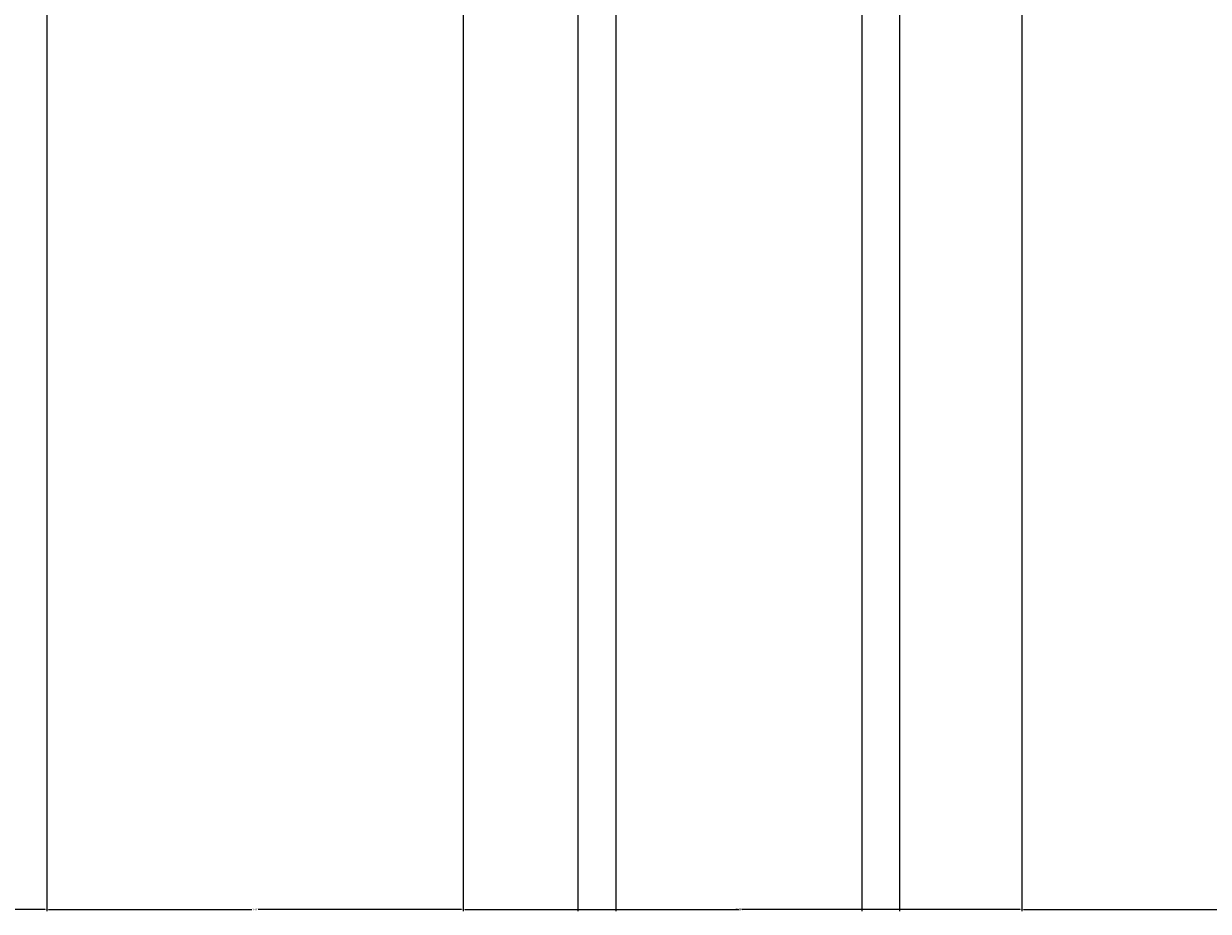
# Model space of a CAD drawing. Units: inches. Extents: x 37 to 824, y -700 to 234.
# Tile 9 of 77: x 253 to 378, y -700 to -606. Entities that reach past the tile are written whole.
import ezdxf

# ---------------------------------------------------------------- set-up
doc = ezdxf.new("R2010")
doc.units = ezdxf.units.IN
doc.header["$MEASUREMENT"] = 0
doc.layers.add('A-ANNO-DIMS', color=2, linetype='Continuous', lineweight=18)
doc.styles.get("Standard").update_dxf_attribs({"font": 'arial.ttf'})
doc.dimstyles.get("Standard").update_dxf_attribs({"dimtxt": 0.18, "dimasz": 0.18, "dimexe": 0.18, "dimexo": 0.0625, "dimgap": 0.09, "dimtad": 0, "dimtih": 1, "dimtoh": 1, "dimdec": 1, "dimzin": 0, "dimdsep": 46, "dimlunit": 4, "dimtxsty": 'Standard', "dimcen": 0.09, "dimadec": 0, "dimazin": 0, "dimtfac": 1, "dimtdec": 1, "dimtofl": 0, "dimtmove": 0, "dimatfit": 3, "dimfxl": 1, "dimtolj": 1, "dimtzin": 0, "dimarcsym": 0})

# ---------------------------------------------------------------- blocks, each defined once
blk = doc.blocks.new('*D68')
at = {"layer": 'A-ANNO-DIMS', "color": 0, "lineweight": -2, "ltscale": 0.5, "transparency": 16777216}
for p, q in [((205.08, -537.69), (205.08, -699.59)), ((255.08, -537.69), (255.08, -699.59)), ((205.26, -699.41), (229.74, -699.41)), ((254.9, -699.41), (230.41, -699.41))]:
    blk.add_line(p, q, dxfattribs=at)
at = {"layer": 'A-ANNO-DIMS', "color": 0, "ltscale": 0.5, "transparency": 16777216}
for points in [[(205.26, -699.38), (205.26, -699.44), (205.08, -699.41)], [(254.9, -699.38), (254.9, -699.44), (255.08, -699.41)]]:
    blk.add_solid(points, dxfattribs=at)
at = {"layer": 'Defpoints', "color": 0, "ltscale": 0.5, "transparency": 16777216}
for p in [(205.08, -537.63), (255.08, -537.63), (255.08, -699.41)]:
    blk.add_point(p, dxfattribs=at)
at = {"layer": 'A-ANNO-DIMS', "color": 0, "ltscale": 0.5, "transparency": 16777216, "insert": (230.08, -699.41), "char_height": 0.18, "attachment_point": 5}
blk.add_mtext('\\A1;4\'-2"', dxfattribs=at)
blk = doc.blocks.new('*D69')
at = {"layer": 'A-ANNO-DIMS', "color": 0, "lineweight": -2, "ltscale": 0.5, "transparency": 16777216}
for p, q in [((255.08, -537.69), (255.08, -699.59)), ((299.08, -585.69), (299.08, -699.59)), ((255.26, -699.41), (276.75, -699.41)), ((298.9, -699.41), (277.41, -699.41))]:
    blk.add_line(p, q, dxfattribs=at)
at = {"layer": 'A-ANNO-DIMS', "color": 0, "ltscale": 0.5, "transparency": 16777216}
for points in [[(255.26, -699.38), (255.26, -699.44), (255.08, -699.41)], [(298.9, -699.38), (298.9, -699.44), (299.08, -699.41)]]:
    blk.add_solid(points, dxfattribs=at)
at = {"layer": 'Defpoints', "color": 0, "ltscale": 0.5, "transparency": 16777216}
for p in [(255.08, -537.63), (299.08, -585.63), (299.08, -699.41)]:
    blk.add_point(p, dxfattribs=at)
at = {"layer": 'A-ANNO-DIMS', "color": 0, "ltscale": 0.5, "transparency": 16777216, "insert": (277.08, -699.41), "char_height": 0.18, "attachment_point": 5}
blk.add_mtext('\\A1;3\'-8"', dxfattribs=at)
blk = doc.blocks.new('*D70')
at = {"layer": 'A-ANNO-DIMS', "color": 0, "lineweight": -2, "ltscale": 0.5, "transparency": 16777216}
for p, q in [((299.08, -585.69), (299.08, -699.59)), ((358.13, -585.69), (358.13, -699.59)), ((299.26, -699.41), (328.2, -699.41)), ((357.95, -699.41), (329.01, -699.41))]:
    blk.add_line(p, q, dxfattribs=at)
at = {"layer": 'A-ANNO-DIMS', "color": 0, "ltscale": 0.5, "transparency": 16777216}
for points in [[(299.26, -699.38), (299.26, -699.44), (299.08, -699.41)], [(357.95, -699.38), (357.95, -699.44), (358.13, -699.41)]]:
    blk.add_solid(points, dxfattribs=at)
at = {"layer": 'Defpoints', "color": 0, "ltscale": 0.5, "transparency": 16777216}
for p in [(299.08, -585.63), (358.13, -585.63), (358.13, -699.41)]:
    blk.add_point(p, dxfattribs=at)
at = {"layer": 'A-ANNO-DIMS', "color": 0, "ltscale": 0.5, "transparency": 16777216, "insert": (328.6, -699.41), "char_height": 0.18, "attachment_point": 5}
blk.add_mtext('\\A1;4\'-11"', dxfattribs=at)
blk = doc.blocks.new('*D71')
at = {"layer": 'A-ANNO-DIMS', "color": 0, "lineweight": -2, "ltscale": 0.5, "transparency": 16777216}
for p, q in [((358.13, -585.69), (358.13, -699.59)), ((428.08, -585.69), (428.08, -699.59)), ((358.31, -699.41), (392.71, -699.41)), ((427.9, -699.41), (393.5, -699.41))]:
    blk.add_line(p, q, dxfattribs=at)
at = {"layer": 'A-ANNO-DIMS', "color": 0, "ltscale": 0.5, "transparency": 16777216}
for points in [[(358.31, -699.38), (358.31, -699.44), (358.13, -699.41)], [(427.9, -699.38), (427.9, -699.44), (428.08, -699.41)]]:
    blk.add_solid(points, dxfattribs=at)
at = {"layer": 'Defpoints', "color": 0, "ltscale": 0.5, "transparency": 16777216}
for p in [(358.13, -585.63), (428.08, -585.63), (428.08, -699.41)]:
    blk.add_point(p, dxfattribs=at)
at = {"layer": 'A-ANNO-DIMS', "color": 0, "ltscale": 0.5, "transparency": 16777216, "insert": (393.1, -699.41), "char_height": 0.18, "attachment_point": 5}
blk.add_mtext('\\A1;5\'-10"', dxfattribs=at)
blk = doc.blocks.new('*D102')
at = {"layer": 'A-ANNO-DIMS', "color": 0, "lineweight": -2, "ltscale": 0.5, "transparency": 16777216}
for p, q in [((311.2, -499.09), (311.2, -699.59)), ((345.2, -499.09), (345.2, -699.59)), ((311.38, -699.41), (327.79, -699.41)), ((345.02, -699.41), (328.6, -699.41))]:
    blk.add_line(p, q, dxfattribs=at)
at = {"layer": 'A-ANNO-DIMS', "color": 0, "ltscale": 0.5, "transparency": 16777216}
for points in [[(311.38, -699.38), (311.38, -699.44), (311.2, -699.41)], [(345.02, -699.38), (345.02, -699.44), (345.2, -699.41)]]:
    blk.add_solid(points, dxfattribs=at)
at = {"layer": 'Defpoints', "color": 0, "ltscale": 0.5, "transparency": 16777216}
for p in [(311.2, -499.03), (345.2, -499.03), (345.2, -699.41)]:
    blk.add_point(p, dxfattribs=at)
at = {"layer": 'A-ANNO-DIMS', "color": 0, "ltscale": 0.5, "transparency": 16777216, "insert": (328.2, -699.41), "char_height": 0.18, "attachment_point": 5}
blk.add_mtext('\\A1;2\'-10"', dxfattribs=at)
blk = doc.blocks.new('*D103')
at = {"layer": 'A-ANNO-DIMS', "color": 0, "lineweight": -2, "ltscale": 0.5, "transparency": 16777216}
for p, q in [((315.2, -505.09), (315.2, -699.59)), ((341.2, -505.09), (341.2, -699.59)), ((315.38, -699.41), (327.86, -699.41)), ((341.02, -699.41), (328.53, -699.41))]:
    blk.add_line(p, q, dxfattribs=at)
at = {"layer": 'A-ANNO-DIMS', "color": 0, "ltscale": 0.5, "transparency": 16777216}
for points in [[(315.38, -699.38), (315.38, -699.44), (315.2, -699.41)], [(341.02, -699.38), (341.02, -699.44), (341.2, -699.41)]]:
    blk.add_solid(points, dxfattribs=at)
at = {"layer": 'Defpoints', "color": 0, "ltscale": 0.5, "transparency": 16777216}
for p in [(315.2, -505.03), (341.2, -505.03), (341.2, -699.41)]:
    blk.add_point(p, dxfattribs=at)
at = {"layer": 'A-ANNO-DIMS', "color": 0, "ltscale": 0.5, "transparency": 16777216, "insert": (328.2, -699.41), "char_height": 0.18, "attachment_point": 5}
blk.add_mtext('\\A1;2\'-2"', dxfattribs=at)

msp = doc.modelspace()

# ---------------------------------------------------------------- dimensions: what is measured, and where the dimension line sits
at = {"layer": 'A-ANNO-DIMS', "ltscale": 0.5}
for base, p1, p2, picture, middle in [((345.2, -699.41), (311.2, -499.03), (345.2, -499.03), '*D102', (328.2, -699.41)), ((341.2, -699.41), (315.2, -505.03), (341.2, -505.03), '*D103', (328.2, -699.41)), ((255.08, -699.41), (205.08, -537.63), (255.08, -537.63), '*D68', (230.08, -699.41)), ((299.08, -699.41), (255.08, -537.63), (299.08, -585.63), '*D69', (277.08, -699.41)), ((358.1323, -699.4145), (299.0772, -585.6275), (358.1323, -585.6275), '*D70', (328.6047, -699.4145)), ((428.0772, -699.4145), (358.1323, -585.6275), (428.0772, -585.6275), '*D71', (393.1047, -699.4145))]:
    dim = msp.add_linear_dim(base=base, p1=p1, p2=p2, dimstyle='Standard', override={"dimdec": 1, "dimlfac": 1, "dimrnd": 0, "dimzin": 1, "dimdsep": 46, "dimlunit": 4, "dimfrac": 2}, dxfattribs=at)
    dim.commit()
    dim.dimension.update_dxf_attribs({"geometry": picture, "text_midpoint": middle})

doc.saveas('drawing.dxf')
